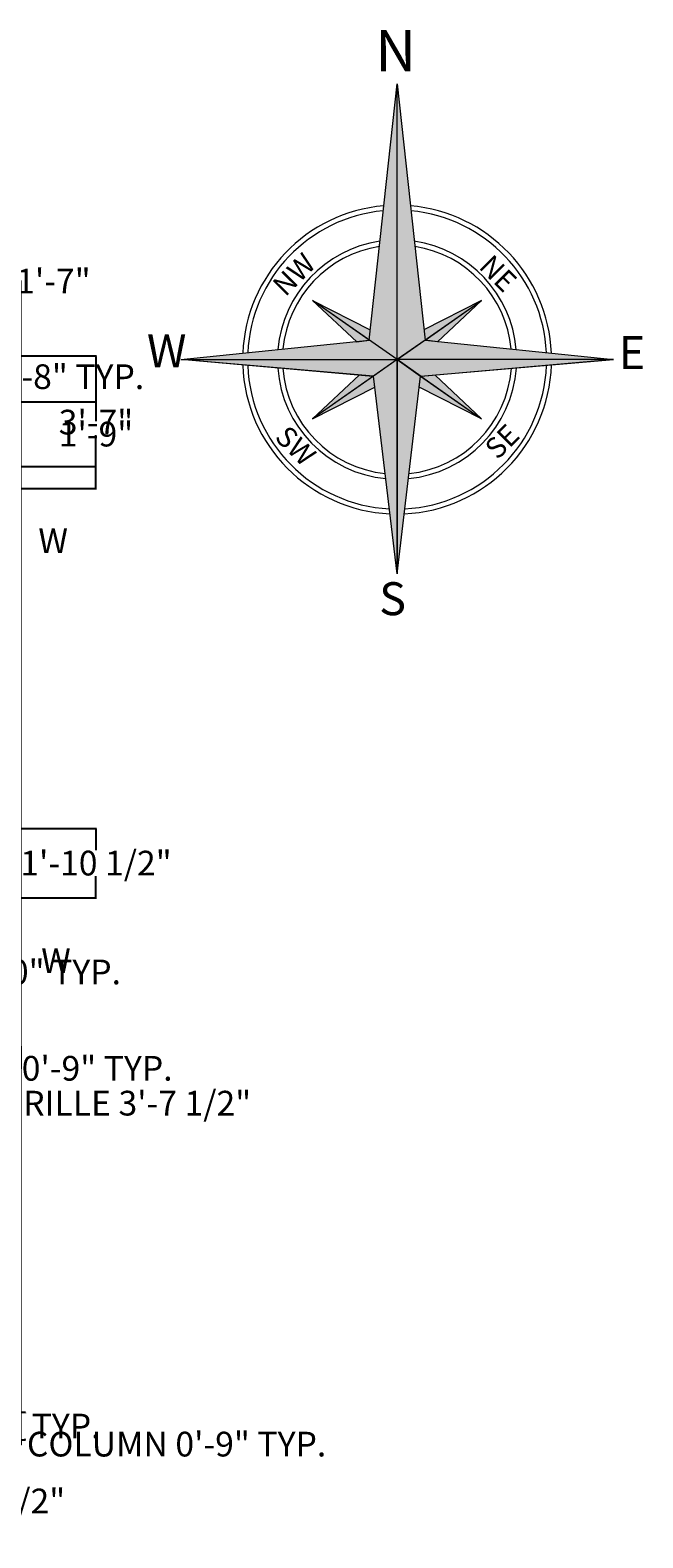
# Model space of a CAD drawing. Units: inches. Extents: x 1305 to 1889, y -508 to -5.
# Tile 8 of 8: x 1691 to 1889, y -493 to -5. Entities that reach past the tile are written whole.
import ezdxf

# ---------------------------------------------------------------- set-up
doc = ezdxf.new("R2010")
doc.units = ezdxf.units.IN
doc.header["$MEASUREMENT"] = 0
for name, color, linetype, lineweight in [('A-ANNO-DIMS', 2, 'Continuous', 18), ('A-ANNO-SYMB', 7, 'Continuous', 18), ('A-ANNO-TEXT', 7, 'Continuous', 18)]:
    doc.layers.add(name, color=color, linetype=linetype, lineweight=lineweight)
doc.styles.get("Standard").update_dxf_attribs({"font": 'arial.ttf', "height": 8})
doc.styles.add('SUPERFRENCH', font='SUF_____.pfb', dxfattribs={"oblique": 15, "height": 2})
doc.dimstyles.get("Standard").update_dxf_attribs({"dimtxt": 0.18, "dimasz": 0.18, "dimexe": 0.18, "dimexo": 0.0625, "dimgap": 0.09, "dimtad": 0, "dimtih": 1, "dimtoh": 1, "dimzin": 0, "dimdsep": 46, "dimlunit": 4, "dimtxsty": 'Standard', "dimcen": 0.09, "dimadec": 0, "dimazin": 0, "dimtfac": 1, "dimtofl": 0, "dimtmove": 0, "dimatfit": 3, "dimfxl": 1, "dimtolj": 1, "dimtzin": 0, "dimarcsym": 0})

# ---------------------------------------------------------------- blocks, each defined once
blk = doc.blocks.new('*D30')
at = {"layer": 'A-ANNO-DIMS', "color": 0, "lineweight": -2, "transparency": 16777216}
for p, q in [((1679.05, -461.36), (1679.05, -462.83)), ((1679.23, -462.65), (1687.87, -462.65)), ((1688.05, -461.36), (1688.05, -462.83)), ((1688.05, -462.65), (1688.23, -462.65))]:
    blk.add_line(p, q, dxfattribs=at)
at = {"layer": 'A-ANNO-DIMS', "color": 0, "transparency": 16777216}
for points in [[(1679.23, -462.62), (1679.23, -462.68), (1679.05, -462.65)], [(1687.87, -462.62), (1687.87, -462.68), (1688.05, -462.65)]]:
    blk.add_solid(points, dxfattribs=at)
at = {"layer": 'Defpoints', "color": 0, "transparency": 16777216}
for p in [(1679.05, -461.3), (1688.05, -461.3), (1688.05, -462.65)]:
    blk.add_point(p, dxfattribs=at)
at = {"layer": 'A-ANNO-DIMS', "color": 0, "transparency": 16777216, "insert": (1738.43, -462.65), "char_height": 8, "attachment_point": 5}
blk.add_mtext('\\A1;COLUMN 0\'-9" TYP.', dxfattribs=at)
blk = doc.blocks.new('*D31')
at = {"layer": 'A-ANNO-DIMS', "color": 0, "lineweight": -2, "transparency": 16777216}
for p, q in [((1688.12, -452.3), (1689.58, -452.3)), ((1689.4, -452.48), (1689.4, -452.62)), ((1688.12, -461.3), (1689.58, -461.3)), ((1689.4, -461.12), (1689.4, -460.97))]:
    blk.add_line(p, q, dxfattribs=at)
at = {"layer": 'A-ANNO-DIMS', "color": 0, "transparency": 16777216}
for points in [[(1689.37, -452.48), (1689.43, -452.48), (1689.4, -452.3)], [(1689.37, -461.12), (1689.43, -461.12), (1689.4, -461.3)]]:
    blk.add_solid(points, dxfattribs=at)
at = {"layer": 'Defpoints', "color": 0, "transparency": 16777216}
for p in [(1688.05, -452.3), (1689.4, -452.3), (1688.05, -461.3)]:
    blk.add_point(p, dxfattribs=at)
at = {"layer": 'A-ANNO-DIMS', "color": 0, "transparency": 16777216, "insert": (1689.4, -456.8), "char_height": 8, "attachment_point": 5}
blk.add_mtext('\\A1;0\'-9" TYP.', dxfattribs=at)
blk = doc.blocks.new('*D32')
at = {"layer": 'A-ANNO-DIMS', "color": 0, "lineweight": -2, "transparency": 16777216}
for p, q in [((1679.01, -285.74), (1671.69, -285.74)), ((1671.87, -285.92), (1671.87, -305.51)), ((1671.87, -333.56), (1671.87, -313.97)), ((1679.01, -333.74), (1671.69, -333.74))]:
    blk.add_line(p, q, dxfattribs=at)
at = {"layer": 'A-ANNO-DIMS', "color": 0, "transparency": 16777216}
for points in [[(1671.84, -285.92), (1671.9, -285.92), (1671.87, -285.74)], [(1671.84, -333.56), (1671.9, -333.56), (1671.87, -333.74)]]:
    blk.add_solid(points, dxfattribs=at)
at = {"layer": 'Defpoints', "color": 0, "transparency": 16777216}
for p in [(1679.07, -285.74), (1671.87, -333.74), (1679.07, -333.74)]:
    blk.add_point(p, dxfattribs=at)
at = {"layer": 'A-ANNO-DIMS', "color": 0, "transparency": 16777216, "insert": (1671.87, -309.74), "char_height": 8, "attachment_point": 5}
blk.add_mtext('\\A1;WINDOW 4\'-0" TYP.', dxfattribs=at)
blk = doc.blocks.new('*D33')
at = {"layer": 'A-ANNO-DIMS', "color": 0, "lineweight": -2, "transparency": 16777216}
for p, q in [((1679.07, -333.8), (1679.07, -341.12)), ((1688.07, -333.8), (1688.07, -341.12)), ((1679.25, -340.94), (1687.89, -340.94)), ((1688.07, -340.94), (1688.25, -340.94))]:
    blk.add_line(p, q, dxfattribs=at)
at = {"layer": 'A-ANNO-DIMS', "color": 0, "transparency": 16777216}
for points in [[(1679.25, -340.91), (1679.25, -340.97), (1679.07, -340.94)], [(1687.89, -340.91), (1687.89, -340.97), (1688.07, -340.94)]]:
    blk.add_solid(points, dxfattribs=at)
at = {"layer": 'Defpoints', "color": 0, "transparency": 16777216}
for p in [(1679.07, -333.74), (1688.07, -333.74), (1688.07, -340.94)]:
    blk.add_point(p, dxfattribs=at)
at = {"layer": 'A-ANNO-DIMS', "color": 0, "transparency": 16777216, "insert": (1712.73, -340.94), "char_height": 8, "attachment_point": 5}
blk.add_mtext('\\A1;0\'-9" TYP.', dxfattribs=at)
blk = doc.blocks.new('*D38')
at = {"layer": 'A-ANNO-DIMS', "color": 0, "lineweight": -2, "transparency": 16777216}
for p, q in [((1591.1, -125.34), (1591.1, -116.79)), ((1591.28, -116.97), (1647.11, -116.97)), ((1647.29, -125.34), (1647.29, -116.79)), ((1647.29, -116.97), (1647.47, -116.97))]:
    blk.add_line(p, q, dxfattribs=at)
at = {"layer": 'A-ANNO-DIMS', "color": 0, "transparency": 16777216}
for points in [[(1591.28, -116.94), (1591.28, -117), (1591.1, -116.97)], [(1647.11, -116.94), (1647.11, -117), (1647.29, -116.97)]]:
    blk.add_solid(points, dxfattribs=at)
at = {"layer": 'Defpoints', "color": 0, "transparency": 16777216}
for p in [(1647.29, -116.97), (1591.1, -125.4), (1647.29, -125.4)]:
    blk.add_point(p, dxfattribs=at)
at = {"layer": 'A-ANNO-DIMS', "color": 0, "transparency": 16777216, "insert": (1688.69, -116.97), "char_height": 8, "attachment_point": 5}
blk.add_mtext('\\A1;SOFA 4\'-8" TYP.', dxfattribs=at)
blk = doc.blocks.new('*D42')
at = {"layer": 'A-ANNO-DIMS', "color": 0, "lineweight": -2, "transparency": 16777216}
for p, q in [((1637.07, -358.66), (1637.07, -352.05)), ((1637.25, -352.23), (1680.16, -352.23)), ((1680.34, -358.66), (1680.34, -352.05)), ((1680.34, -352.23), (1680.52, -352.23))]:
    blk.add_line(p, q, dxfattribs=at)
at = {"layer": 'A-ANNO-DIMS', "color": 0, "transparency": 16777216}
for points in [[(1637.25, -352.2), (1637.25, -352.26), (1637.07, -352.23)], [(1680.16, -352.2), (1680.16, -352.26), (1680.34, -352.23)]]:
    blk.add_solid(points, dxfattribs=at)
at = {"layer": 'Defpoints', "color": 0, "transparency": 16777216}
for p in [(1680.34, -352.23), (1637.07, -358.72), (1680.34, -358.72)]:
    blk.add_point(p, dxfattribs=at)
at = {"layer": 'A-ANNO-DIMS', "color": 0, "transparency": 16777216, "insert": (1721.92, -352.23), "char_height": 8, "attachment_point": 5}
blk.add_mtext('\\A1;GRILLE 3\'-7 1/2"', dxfattribs=at)
blk = doc.blocks.new('*D54')
at = {"layer": 'A-ANNO-DIMS', "color": 0, "lineweight": -2, "transparency": 16777216}
for p, q in [((1544.74, -125.07), (1712.53, -125.07)), ((1712.35, -125.25), (1712.35, -131.39)), ((1712.35, -145.89), (1712.35, -139.74)), ((1544.74, -146.07), (1712.53, -146.07))]:
    blk.add_line(p, q, dxfattribs=at)
at = {"layer": 'A-ANNO-DIMS', "color": 0, "transparency": 16777216}
for points in [[(1712.32, -125.25), (1712.38, -125.25), (1712.35, -125.07)], [(1712.32, -145.89), (1712.38, -145.89), (1712.35, -146.07)]]:
    blk.add_solid(points, dxfattribs=at)
at = {"layer": 'Defpoints', "color": 0, "transparency": 16777216}
for p in [(1544.68, -125.07), (1544.68, -146.07), (1712.35, -146.07)]:
    blk.add_point(p, dxfattribs=at)
at = {"layer": 'A-ANNO-DIMS', "color": 0, "transparency": 16777216, "insert": (1712.35, -135.57), "char_height": 8, "attachment_point": 5}
blk.add_mtext('\\A1;1\'-9"', dxfattribs=at)
blk = doc.blocks.new('*D64')
at = {"layer": 'A-ANNO-DIMS', "color": 0, "lineweight": -2, "transparency": 16777216}
for p, q in [((1669.29, -461.18), (1669.29, -85.83)), ((1669.47, -86.01), (1687.87, -86.01)), ((1688.05, -461.23), (1688.05, -85.83)), ((1688.05, -86.01), (1688.23, -86.01))]:
    blk.add_line(p, q, dxfattribs=at)
at = {"layer": 'A-ANNO-DIMS', "color": 0, "transparency": 16777216}
for points in [[(1669.47, -85.98), (1669.47, -86.04), (1669.29, -86.01)], [(1687.87, -85.98), (1687.87, -86.04), (1688.05, -86.01)]]:
    blk.add_solid(points, dxfattribs=at)
at = {"layer": 'Defpoints', "color": 0, "transparency": 16777216}
for p in [(1688.05, -86.01), (1669.29, -461.24), (1688.05, -461.3)]:
    blk.add_point(p, dxfattribs=at)
at = {"layer": 'A-ANNO-DIMS', "color": 0, "transparency": 16777216, "insert": (1698.58, -86.01), "char_height": 8, "attachment_point": 5}
blk.add_mtext('\\A1;1\'-7"', dxfattribs=at)
blk = doc.blocks.new('*D67')
at = {"layer": 'A-ANNO-DIMS', "color": 0, "lineweight": -2, "transparency": 16777216}
for p, q in [((1688.14, -110.24), (1712.53, -110.24)), ((1712.35, -110.42), (1712.35, -127.51)), ((1712.35, -152.96), (1712.35, -135.87)), ((1688.14, -153.14), (1712.53, -153.14))]:
    blk.add_line(p, q, dxfattribs=at)
at = {"layer": 'A-ANNO-DIMS', "color": 0, "transparency": 16777216}
for points in [[(1712.32, -110.42), (1712.38, -110.42), (1712.35, -110.24)], [(1712.32, -152.96), (1712.38, -152.96), (1712.35, -153.14)]]:
    blk.add_solid(points, dxfattribs=at)
at = {"layer": 'Defpoints', "color": 0, "transparency": 16777216}
for p in [(1688.07, -110.24), (1688.07, -153.14), (1712.35, -153.14)]:
    blk.add_point(p, dxfattribs=at)
at = {"layer": 'A-ANNO-DIMS', "color": 0, "transparency": 16777216, "insert": (1712.35, -131.69), "char_height": 8, "attachment_point": 5}
blk.add_mtext('\\A1;3\'-7"', dxfattribs=at)
blk = doc.blocks.new('*D68')
at = {"layer": 'A-ANNO-DIMS', "color": 0, "lineweight": -2, "transparency": 16777216}
for p, q in [((1679.14, -263.24), (1712.53, -263.24)), ((1712.35, -263.42), (1712.35, -270.26)), ((1712.35, -285.56), (1712.35, -278.71)), ((1679.14, -285.74), (1712.53, -285.74))]:
    blk.add_line(p, q, dxfattribs=at)
at = {"layer": 'A-ANNO-DIMS', "color": 0, "transparency": 16777216}
for points in [[(1712.32, -263.42), (1712.38, -263.42), (1712.35, -263.24)], [(1712.32, -285.56), (1712.38, -285.56), (1712.35, -285.74)]]:
    blk.add_solid(points, dxfattribs=at)
at = {"layer": 'Defpoints', "color": 0, "transparency": 16777216}
for p in [(1679.07, -263.24), (1679.07, -285.74), (1712.35, -285.74)]:
    blk.add_point(p, dxfattribs=at)
at = {"layer": 'A-ANNO-DIMS', "color": 0, "transparency": 16777216, "insert": (1712.35, -274.49), "char_height": 8, "attachment_point": 5}
blk.add_mtext('\\A1;1\'-10 1/2"', dxfattribs=at)
blk = doc.blocks.new('*D74')
at = {"layer": 'A-ANNO-DIMS', "color": 0, "lineweight": -2, "transparency": 16777216}
for p, q in [((1653.32, -448.48), (1653.5, -448.48)), ((1653.41, -448.57), (1653.41, -448.39)), ((1653.41, -481.07), (1653.41, -469.03)), ((1653.59, -481.07), (1653.41, -481.07))]:
    blk.add_line(p, q, dxfattribs=at)
at = {"layer": 'A-ANNO-DIMS', "color": 0, "transparency": 16777216}
blk.add_solid([(1653.44, -469.03), (1653.38, -469.03), (1653.41, -468.85)], dxfattribs=at)
at = {"layer": 'Defpoints', "color": 0, "transparency": 16777216}
for p in [(1653.41, -448.48), (1653.41, -468.85)]:
    blk.add_point(p, dxfattribs=at)
at = {"layer": 'A-ANNO-DIMS', "color": 0, "transparency": 16777216, "insert": (1677.46, -481.07), "char_height": 8, "attachment_point": 5}
blk.add_mtext('\\A1;R1\'-8 1/2"', dxfattribs=at)

msp = doc.modelspace()

# ---------------------------------------------------------------- linework, layer by layer
at = {"layer": 'A-ANNO-SYMB'}
for p, q in [((1800.75, -105.11), (1809.795, -22.089)), ((1809.795, -180.792), (1809.795, -22.089)), ((1809.795, -180.792), (1809.795, -22.089)), ((1809.795, -111.443), (1809.795, -22.089)), ((1809.795, -22.089), (1818.841, -105.11)), ((1809.795, -22.089), (1818.841, -105.11)), ((1809.795, -111.443), (1782.456, -92.3)), ((1782.456, -92.3), (1796.727, -105.676)), ((1782.456, -92.3), (1801.117, -101.748)), ((1800.75, -105.11), (1782.456, -92.3)), ((1782.456, -92.3), (1796.727, -105.676)), ((1809.795, -111.443), (1837.135, -92.3)), ((1837.135, -92.3), (1818.474, -101.748)), ((1818.841, -105.11), (1837.135, -92.3)), ((1837.135, -92.3), (1822.864, -105.676)), ((1837.135, -92.3), (1822.864, -105.676)), ((1739.779, -111.443), (1800.75, -105.11)), ((1796.727, -105.676), (1800.75, -105.11)), ((1818.841, -105.11), (1809.795, -111.443)), ((1822.864, -105.676), (1818.841, -105.11)), ((1818.841, -105.11), (1879.812, -111.443)), ((1739.779, -111.443), (1809.795, -111.443)), ((1739.779, -111.443), (1809.795, -111.443)), ((1802.202, -116.76), (1739.779, -111.443)), ((1801.982, -116.914), (1739.779, -111.443)), ((1809.795, -111.443), (1782.456, -130.586)), ((1809.795, -111.443), (1802.202, -116.76)), ((1809.795, -111.443), (1837.135, -130.586)), ((1879.812, -111.443), (1809.795, -111.443)), ((1879.812, -111.443), (1809.795, -111.443)), ((1809.795, -111.443), (1817.389, -116.76)), ((1817.609, -116.914), (1809.795, -111.443)), ((1809.795, -111.443), (1809.795, -180.792)), ((1817.389, -116.76), (1879.812, -111.443)), ((1879.812, -111.443), (1817.609, -116.914)), ((1782.456, -130.586), (1797.623, -116.37)), ((1802.202, -116.76), (1782.456, -130.586)), ((1802.63, -120.372), (1802.202, -116.76)), ((1809.795, -180.792), (1802.202, -116.76)), ((1809.795, -180.792), (1817.389, -116.76)), ((1816.961, -120.372), (1817.389, -116.76)), ((1817.389, -116.76), (1837.135, -130.586)), ((1837.135, -130.586), (1822.124, -116.517)), ((1782.456, -130.586), (1802.63, -120.372)), ((1782.456, -130.586), (1802.63, -120.372)), ((1837.135, -130.586), (1816.961, -120.372)), ((1837.135, -130.586), (1816.961, -120.372))]:
    msp.add_line(p, q, dxfattribs=at)
for radius, start, end in [(49.997, 94.94314, 177.61114), (48.385, 95.3202, 177.33176), (49.997, 2.38886, 85.05686), (48.385, 2.66824, 84.6798), (38.708, 98.26104, 175.15907), (38.708, 4.84093, 81.73896), (37.095, 98.90525, 174.68478), (37.095, 5.31522, 81.09475), (49.997, 182.02127, 267.36189), (48.385, 182.25745, 267.04553), (38.708, 184.09236, 264.58271), (37.095, 184.49244, 264.04444), (49.997, 272.63811, 357.97873), (48.385, 272.95447, 357.74255), (38.708, 275.41729, 355.90764), (37.095, 275.95556, 355.50756)]:
    msp.add_arc((1809.795, -111.443), radius, start, end, dxfattribs=at)
for points in [[(1806.78, -79.547), (1809.795, -22.089), (1800.75, -105.11)], [(1806.78, -79.547), (1809.795, -111.443), (1809.795, -22.089)], [(1809.795, -22.089), (1809.795, -111.443), (1818.841, -105.11)], [(1806.78, -79.547), (1800.75, -105.11), (1809.795, -111.443)], [(1782.456, -92.3), (1796.585, -105.542), (1800.75, -105.11)], [(1782.456, -92.3), (1800.75, -105.11), (1801.117, -101.748)], [(1818.474, -101.748), (1818.841, -105.11), (1837.135, -92.3)], [(1818.841, -105.11), (1823.006, -105.542), (1837.135, -92.3)], [(1739.779, -111.443), (1796.727, -105.676), (1796.585, -105.542)], [(1739.779, -111.443), (1809.795, -111.443), (1796.727, -105.676)], [(1796.727, -105.676), (1809.795, -111.443), (1800.75, -105.11)], [(1809.795, -111.443), (1822.864, -105.676), (1818.841, -105.11)], [(1809.795, -111.443), (1879.812, -111.443), (1822.864, -105.676)], [(1822.864, -105.676), (1879.812, -111.443), (1823.006, -105.542)], [(1739.779, -111.443), (1802.202, -116.76), (1809.795, -111.443)], [(1809.795, -111.443), (1802.202, -116.76), (1809.795, -180.792)], [(1809.795, -111.443), (1817.389, -116.76), (1879.812, -111.443)], [(1817.389, -116.76), (1809.795, -111.443), (1809.795, -180.792)], [(1782.456, -130.586), (1801.982, -116.914), (1797.467, -116.517)], [(1782.456, -130.586), (1802.63, -120.372), (1802.202, -116.76)], [(1817.389, -116.76), (1816.961, -120.372), (1837.135, -130.586)], [(1817.609, -116.914), (1837.135, -130.586), (1822.124, -116.517)]]:
    msp.add_solid(points, dxfattribs=at)

# ---------------------------------------------------------------- texts
at = {"layer": 'A-ANNO-SYMB', "style": 'SUPERFRENCH', "oblique": 15}
for s, height, p in [('N', 13.336, (1802.763, -18.088)), ('W', 10.669, (1728.844, -113.977)), ('E', 10.669, (1881.545, -114.51)), ('S', 10.669, (1803.997, -194.199))]:
    msp.add_text(s, height=height, dxfattribs=at).set_placement(p)
for s, rotation, p in [('NW', 45, (1773.623, -91.37)), ('NE', 315, (1835.934, -81.643)), ('SW', 315, (1769.878, -136.967)), ('SE', 45, (1842.289, -144.132))]:
    msp.add_text(s, height=6.6682, rotation=rotation, dxfattribs=at).set_placement(p)
at = {"layer": 'A-ANNO-TEXT', "char_height": 8, "attachment_point": 1}
for insert in [(1693.69, -166.115), (1694.613, -302.065)]:
    msp.add_mtext_dynamic_manual_height_columns('W', width=13.3749, gutter_width=40, heights=[0], dxfattribs=dict(at, insert=insert))

# ---------------------------------------------------------------- dimensions: what is measured, and where the dimension line sits
at = {"layer": 'A-ANNO-DIMS'}
dim = msp.add_linear_dim(base=(1688.053, -86.014), p1=(1669.285, -461.239), p2=(1688.053, -461.295), dimstyle='Standard', override={"dimdec": 1, "dimlfac": 1, "dimrnd": 0, "dimzin": 1, "dimdsep": 46, "dimlunit": 4, "dimfrac": 2}, dxfattribs=at)
dim.commit()
dim.dimension.update_dxf_attribs({"geometry": '*D64', "text_midpoint": (1698.58, -86.014)})
for base, p1, p2, text, picture, middle in [((1647.29, -116.975), (1591.1, -125.403), (1647.29, -125.403), 'SOFA <> TYP.', '*D38', (1688.69, -116.975)), ((1688.074, -340.939), (1679.074, -333.739), (1688.074, -333.739), '<> TYP.', '*D33', (1712.726, -340.939)), ((1680.336, -352.234), (1637.074, -358.723), (1680.336, -358.723), 'GRILLE <>', '*D42', (1721.924, -352.234)), ((1688.053, -462.645), (1679.053, -461.295), (1688.053, -461.295), 'COLUMN <> TYP.', '*D30', (1738.427, -462.645))]:
    dim = msp.add_linear_dim(base=base, p1=p1, p2=p2, text=text, dimstyle='Standard', override={"dimdec": 1, "dimlfac": 1, "dimrnd": 0, "dimzin": 1, "dimdsep": 46, "dimlunit": 4, "dimfrac": 2}, dxfattribs=at)
    dim.commit()
    dim.dimension.update_dxf_attribs({"geometry": picture, "text_midpoint": middle})
for base, p1, p2, picture, middle in [((1712.353, -153.14), (1688.074, -110.239), (1688.074, -153.14), '*D67', (1712.353, -131.689)), ((1712.353, -146.069), (1544.679, -125.069), (1544.679, -146.069), '*D54', (1712.353, -135.569)), ((1712.353, -285.739), (1679.074, -263.239), (1679.074, -285.739), '*D68', (1712.353, -274.489))]:
    dim = msp.add_linear_dim(base=base, p1=p1, p2=p2, angle=90, dimstyle='Standard', override={"dimdec": 1, "dimlfac": 1, "dimrnd": 0, "dimzin": 1, "dimdsep": 46, "dimlunit": 4, "dimfrac": 2}, dxfattribs=at)
    dim.commit()
    dim.dimension.update_dxf_attribs({"geometry": picture, "text_midpoint": middle})
for base, p1, p2, angle, text, picture, middle in [((1671.874, -333.739), (1679.074, -285.739), (1679.074, -333.739), 270, 'WINDOW <> TYP.', '*D32', (1671.874, -309.739)), ((1689.403, -452.295), (1688.053, -461.295), (1688.053, -452.295), 90, '<> TYP.', '*D31', (1689.403, -456.795))]:
    dim = msp.add_linear_dim(base=base, p1=p1, p2=p2, angle=angle, text=text, dimstyle='Standard', override={"dimdec": 1, "dimlfac": 1, "dimrnd": 0, "dimzin": 1, "dimdsep": 46, "dimlunit": 4, "dimfrac": 2}, dxfattribs=at)
    dim.commit()
    dim.dimension.update_dxf_attribs({"geometry": picture, "text_midpoint": middle})
dim = msp.add_radius_dim(center=(1653.406, -448.483), mpoint=(1653.406, -468.851), dimstyle='Standard', override={"dimdec": 1, "dimlfac": 1, "dimrnd": 0, "dimzin": 1, "dimdsep": 46, "dimlunit": 4, "dimfrac": 2}, dxfattribs=at)
dim.commit()
dim.dimension.update_dxf_attribs({"geometry": '*D74', "text_midpoint": (1677.458, -481.072), "dimtype": 164})

doc.saveas('drawing.dxf')
